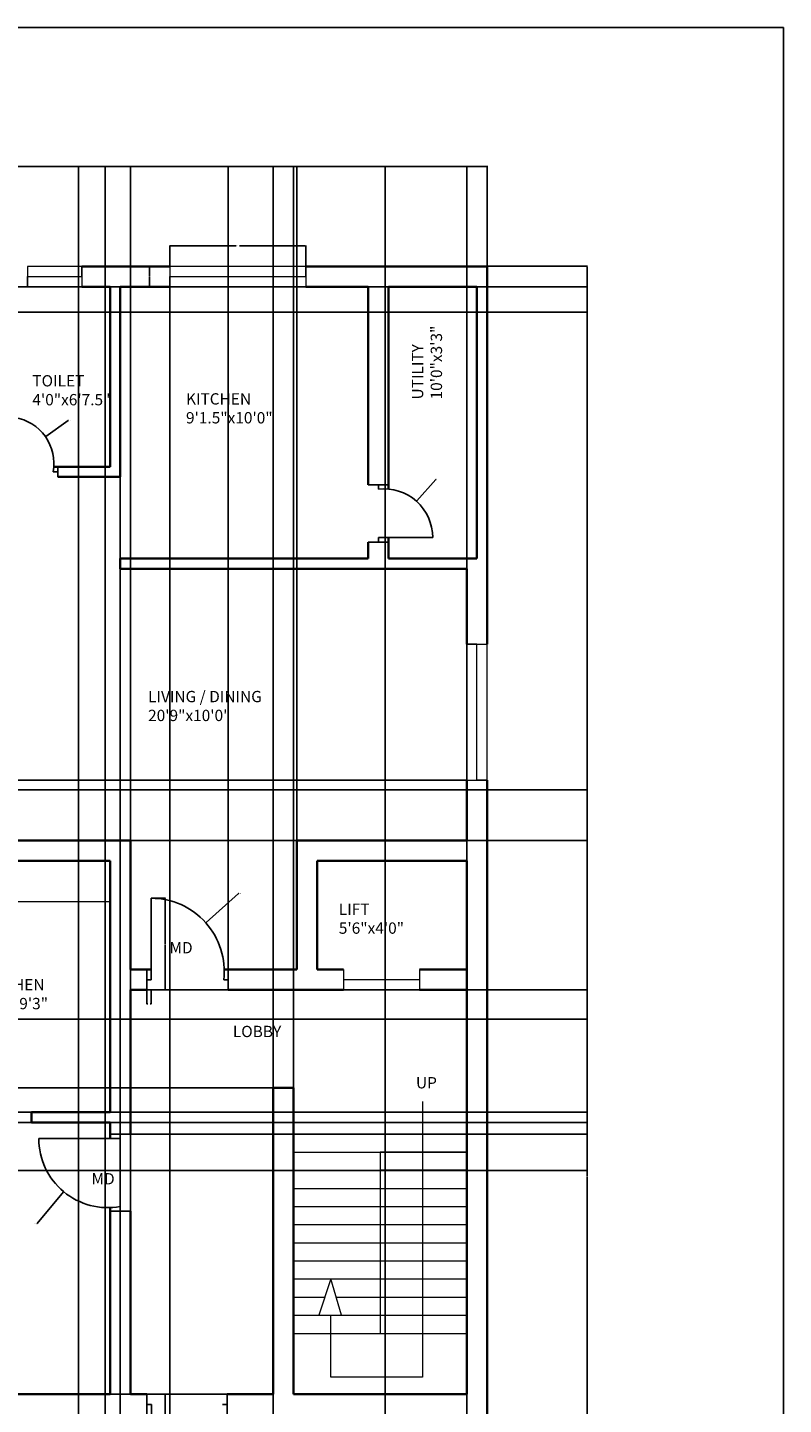
# Model space of a CAD drawing. Units: inches. Extents: x 1870 to 2611, y 1432 to 2511.
# Tile 5 of 5: x 2277 to 2611, y 1903 to 2511. Entities that reach past the tile are written whole.
import ezdxf

# ---------------------------------------------------------------- set-up
doc = ezdxf.new("R2010")
doc.units = ezdxf.units.IN
for name, color, linetype, lineweight in [('A-ANNO-DIMS', 2, 'Continuous', 18), ('A-ANNO-SYMB', 60, 'Continuous', 18), ('A-ANNO-TEXT', 7, 'Continuous', 18), ('A-ANNO-TTLB', 7, 'Continuous', 25), ('A-AREA-IDEN', 7, 'Continuous', 18), ('A-DOOR', 31, 'Continuous', 25), ('A-EQPM-ELEV', 4, 'Continuous', 18), ('A-FLOR-FIXT', 8, 'Continuous', 18), ('A-FLOR-STRS', 60, 'Continuous', 18), ('A-GLAZ', 201, 'Continuous', 18), ('A-WALL', 7, 'Continuous', 35)]:
    doc.layers.add(name, color=color, linetype=linetype, lineweight=lineweight)
doc.styles.get("Standard").update_dxf_attribs({"font": 'arial.ttf'})
doc.dimstyles.get("Standard").update_dxf_attribs({"dimtxt": 0.18, "dimasz": 0.18, "dimexe": 0.18, "dimexo": 0.0625, "dimgap": 0.09, "dimtad": 0, "dimtih": 1, "dimtoh": 1, "dimdec": 4, "dimzin": 0, "dimdsep": 46, "dimtxsty": 'Standard', "dimcen": 0.09, "dimadec": 0, "dimazin": 0, "dimtfac": 1, "dimtdec": 4, "dimtofl": 0, "dimtmove": 0, "dimatfit": 3, "dimfxl": 1, "dimtolj": 1, "dimtzin": 0, "dimarcsym": 0})

# ---------------------------------------------------------------- blocks, each defined once
blk = doc.blocks.new('DOOR-LEAF-36-JAMB-9-A')
for p, q in [((2, 4.5), (2, 40.5)), ((0, 9), (0, 0)), ((0, 0), (0, 4.5)), ((0, 4.5), (2, 4.5))]:
    blk.add_line(p, q)
blk = doc.blocks.new('DOOR-LEAF-36-JAMB-9-B')
for p, q in [((0, 40.5), (0, 31.5)), ((0, 31.5), (0, 36)), ((0, 36), (2, 36)), ((2, 36), (2, 0))]:
    blk.add_line(p, q)
blk = doc.blocks.new('WIN-60-FRAME-9')
for p, q in [((0, 9), (0, 0)), ((60, 9), (0, 9)), ((60, 4.5), (60, 9)), ((60, 9), (60, 0)), ((0, 0), (0, 4.5)), ((0, 4.5), (60, 4.5)), ((0, 0), (60, 0))]:
    blk.add_line(p, q)
blk = doc.blocks.new('WIN-24-FRAME-9')
for p, q in [((0, 9), (0, 0)), ((24, 9), (0, 9)), ((24, 4.5), (24, 9)), ((24, 9), (24, 0)), ((0, 0), (0, 4.5)), ((0, 4.5), (24, 4.5)), ((0, 0), (24, 0))]:
    blk.add_line(p, q)
blk = doc.blocks.new('*D11')
at = {"layer": 'A-ANNO-DIMS', "color": 0, "lineweight": -2, "transparency": 16777216}
for p, q in [((2340.04, 2405.43), (2340.04, 2414.55)), ((2340.22, 2414.37), (2369.28, 2414.37)), ((2399.86, 2414.37), (2370.79, 2414.37)), ((2400.04, 2405.43), (2400.04, 2414.55))]:
    blk.add_line(p, q, dxfattribs=at)
at = {"layer": 'A-ANNO-DIMS', "color": 0, "transparency": 16777216}
for points in [[(2340.22, 2414.4), (2340.22, 2414.34), (2340.04, 2414.37)], [(2399.86, 2414.4), (2399.86, 2414.34), (2400.04, 2414.37)]]:
    blk.add_solid(points, dxfattribs=at)
at = {"layer": 'Defpoints', "color": 0, "transparency": 16777216}
for p in [(2400.04, 2414.37), (2340.04, 2405.37), (2400.04, 2405.37)]:
    blk.add_point(p, dxfattribs=at)
at = {"layer": 'A-ANNO-DIMS', "color": 0, "transparency": 16777216, "insert": (2370.04, 2414.37), "char_height": 0.18, "attachment_point": 5}
blk.add_mtext('\\A1;W1 60 TYP.', dxfattribs=at)
blk = doc.blocks.new('*D12')
at = {"layer": 'A-ANNO-DIMS', "color": 0, "lineweight": -2, "transparency": 16777216}
for p, q in [((2339.97, 2405.37), (2330.86, 2405.37)), ((2331.04, 2405.19), (2331.04, 2401.05)), ((2339.97, 2396.37), (2330.86, 2396.37)), ((2331.04, 2396.55), (2331.04, 2400.69))]:
    blk.add_line(p, q, dxfattribs=at)
at = {"layer": 'A-ANNO-DIMS', "color": 0, "transparency": 16777216}
for points in [[(2331.01, 2405.19), (2331.07, 2405.19), (2331.04, 2405.37)], [(2331.01, 2396.55), (2331.07, 2396.55), (2331.04, 2396.37)]]:
    blk.add_solid(points, dxfattribs=at)
at = {"layer": 'Defpoints', "color": 0, "transparency": 16777216}
for p in [(2331.04, 2405.37), (2340.04, 2405.37), (2340.04, 2396.37)]:
    blk.add_point(p, dxfattribs=at)
at = {"layer": 'A-ANNO-DIMS', "color": 0, "transparency": 16777216, "insert": (2331.04, 2400.87), "char_height": 0.18, "attachment_point": 5}
blk.add_mtext('\\A1;9 TYP.', dxfattribs=at)
blk = doc.blocks.new('*D19')
at = {"layer": 'A-ANNO-DIMS', "color": 0, "lineweight": -2, "transparency": 16777216}
for p, q in [((2331.88, 2126.37), (2338.08, 2126.37)), ((2337.9, 2126.19), (2337.9, 2106.3)), ((2337.9, 2086.05), (2337.9, 2105.93)), ((2331.88, 2085.87), (2338.08, 2085.87))]:
    blk.add_line(p, q, dxfattribs=at)
at = {"layer": 'A-ANNO-DIMS', "color": 0, "transparency": 16777216}
for points in [[(2337.87, 2126.19), (2337.93, 2126.19), (2337.9, 2126.37)], [(2337.87, 2086.05), (2337.93, 2086.05), (2337.9, 2085.87)]]:
    blk.add_solid(points, dxfattribs=at)
at = {"layer": 'Defpoints', "color": 0, "transparency": 16777216}
for p in [(2331.82, 2126.37), (2337.9, 2126.37), (2331.82, 2085.87)]:
    blk.add_point(p, dxfattribs=at)
at = {"layer": 'A-ANNO-DIMS', "color": 0, "transparency": 16777216, "insert": (2337.9, 2106.12), "char_height": 0.18, "attachment_point": 5}
blk.add_mtext('\\A1;DOOR C 41 TYP.', dxfattribs=at)
blk = doc.blocks.new('*D20')
at = {"layer": 'A-ANNO-DIMS', "color": 0, "lineweight": -2, "transparency": 16777216}
for p, q in [((2329.82, 2085.8), (2329.82, 2079.61)), ((2331.82, 2085.8), (2331.82, 2079.61)), ((2330, 2079.79), (2330.36, 2079.79)), ((2331.64, 2079.79), (2331.28, 2079.79))]:
    blk.add_line(p, q, dxfattribs=at)
at = {"layer": 'A-ANNO-DIMS', "color": 0, "transparency": 16777216}
for points in [[(2330, 2079.82), (2330, 2079.76), (2329.82, 2079.79)], [(2331.64, 2079.82), (2331.64, 2079.76), (2331.82, 2079.79)]]:
    blk.add_solid(points, dxfattribs=at)
at = {"layer": 'Defpoints', "color": 0, "transparency": 16777216}
for p in [(2329.82, 2085.87), (2331.82, 2085.87), (2331.82, 2079.79)]:
    blk.add_point(p, dxfattribs=at)
at = {"layer": 'A-ANNO-DIMS', "color": 0, "transparency": 16777216, "insert": (2330.82, 2079.79), "char_height": 0.18, "attachment_point": 5}
blk.add_mtext('\\A1;2 TYP.', dxfattribs=at)
blk = doc.blocks.new('*D21')
at = {"layer": 'A-ANNO-DIMS', "color": 0, "lineweight": -2, "transparency": 16777216}
for p, q in [((2331.96, 1907.37), (2338.15, 1907.37)), ((2337.97, 1907.19), (2337.97, 1887.3)), ((2337.97, 1867.05), (2337.97, 1886.93)), ((2331.96, 1866.87), (2338.15, 1866.87))]:
    blk.add_line(p, q, dxfattribs=at)
at = {"layer": 'A-ANNO-DIMS', "color": 0, "transparency": 16777216}
for points in [[(2337.94, 1907.19), (2338, 1907.19), (2337.97, 1907.37)], [(2337.94, 1867.05), (2338, 1867.05), (2337.97, 1866.87)]]:
    blk.add_solid(points, dxfattribs=at)
at = {"layer": 'Defpoints', "color": 0, "transparency": 16777216}
for p in [(2331.9, 1907.37), (2337.97, 1907.37), (2331.9, 1866.87)]:
    blk.add_point(p, dxfattribs=at)
at = {"layer": 'A-ANNO-DIMS', "color": 0, "transparency": 16777216, "insert": (2337.97, 1887.12), "char_height": 0.18, "attachment_point": 5}
blk.add_mtext('\\A1;DOOR D 41 TYP.', dxfattribs=at)
blk = doc.blocks.new('*D25')
at = {"layer": 'A-ANNO-DIMS', "color": 0, "lineweight": -2, "transparency": 16777216}
for p, q in [((2004.64, 2405.43), (2004.64, 2449.7)), ((2004.82, 2449.52), (2241.99, 2449.52)), ((2479.96, 2449.52), (2242.78, 2449.52)), ((2480.14, 2405.43), (2480.14, 2449.7))]:
    blk.add_line(p, q, dxfattribs=at)
at = {"layer": 'A-ANNO-DIMS', "color": 0, "transparency": 16777216}
for points in [[(2004.82, 2449.55), (2004.82, 2449.49), (2004.64, 2449.52)], [(2479.96, 2449.55), (2479.96, 2449.49), (2480.14, 2449.52)]]:
    blk.add_solid(points, dxfattribs=at)
at = {"layer": 'Defpoints', "color": 0, "transparency": 16777216}
for p in [(2480.14, 2449.52), (2004.64, 2405.37), (2480.14, 2405.37)]:
    blk.add_point(p, dxfattribs=at)
at = {"layer": 'A-ANNO-DIMS', "color": 0, "transparency": 16777216, "insert": (2242.39, 2449.52), "char_height": 0.18, "attachment_point": 5}
blk.add_mtext('\\A1;475.5', dxfattribs=at)
blk = doc.blocks.new('*D26')
at = {"layer": 'A-ANNO-DIMS', "color": 0, "lineweight": -2, "transparency": 16777216}
for p, q in [((2480.2, 2405.37), (2524.47, 2405.37)), ((2524.29, 2405.19), (2524.29, 2003.55)), ((2524.29, 1601.55), (2524.29, 2003.19)), ((2480.2, 1601.37), (2524.47, 1601.37))]:
    blk.add_line(p, q, dxfattribs=at)
at = {"layer": 'A-ANNO-DIMS', "color": 0, "transparency": 16777216}
for points in [[(2524.26, 2405.19), (2524.32, 2405.19), (2524.29, 2405.37)], [(2524.26, 1601.55), (2524.32, 1601.55), (2524.29, 1601.37)]]:
    blk.add_solid(points, dxfattribs=at)
at = {"layer": 'Defpoints', "color": 0, "transparency": 16777216}
for p in [(2480.14, 2405.37), (2480.14, 1601.37), (2524.29, 1601.37)]:
    blk.add_point(p, dxfattribs=at)
at = {"layer": 'A-ANNO-DIMS', "color": 0, "transparency": 16777216, "insert": (2524.29, 2003.37), "char_height": 0.18, "attachment_point": 5}
blk.add_mtext('\\A1;804', dxfattribs=at)
blk = doc.blocks.new('*D33')
at = {"layer": 'A-ANNO-DIMS', "color": 0, "lineweight": -2, "transparency": 16777216}
for p, q in [((2394.64, 1907.43), (2394.64, 2449.7)), ((2394.82, 2449.52), (2432.56, 2449.52)), ((2470.96, 2449.52), (2433.21, 2449.52)), ((2471.14, 1907.43), (2471.14, 2449.7))]:
    blk.add_line(p, q, dxfattribs=at)
at = {"layer": 'A-ANNO-DIMS', "color": 0, "transparency": 16777216}
for points in [[(2394.82, 2449.55), (2394.82, 2449.49), (2394.64, 2449.52)], [(2470.96, 2449.55), (2470.96, 2449.49), (2471.14, 2449.52)]]:
    blk.add_solid(points, dxfattribs=at)
at = {"layer": 'Defpoints', "color": 0, "transparency": 16777216}
for p in [(2471.14, 2449.52), (2394.64, 1907.37), (2471.14, 1907.37)]:
    blk.add_point(p, dxfattribs=at)
at = {"layer": 'A-ANNO-DIMS', "color": 0, "transparency": 16777216, "insert": (2432.89, 2449.52), "char_height": 0.18, "attachment_point": 5}
blk.add_mtext('\\A1;76.5', dxfattribs=at)
blk = doc.blocks.new('*D34')
at = {"layer": 'A-ANNO-DIMS', "color": 0, "lineweight": -2, "transparency": 16777216}
for p, q in [((2385.57, 2042.61), (1960.31, 2042.61)), ((1960.49, 2042.43), (1960.49, 1975.17)), ((1960.49, 1907.55), (1960.49, 1974.8)), ((2385.57, 1907.37), (1960.31, 1907.37))]:
    blk.add_line(p, q, dxfattribs=at)
at = {"layer": 'A-ANNO-DIMS', "color": 0, "transparency": 16777216}
for points in [[(1960.46, 2042.43), (1960.52, 2042.43), (1960.49, 2042.61)], [(1960.46, 1907.55), (1960.52, 1907.55), (1960.49, 1907.37)]]:
    blk.add_solid(points, dxfattribs=at)
at = {"layer": 'Defpoints', "color": 0, "transparency": 16777216}
for p in [(1960.49, 2042.61), (2385.64, 2042.61), (2385.64, 1907.37)]:
    blk.add_point(p, dxfattribs=at)
at = {"layer": 'A-ANNO-DIMS', "color": 0, "transparency": 16777216, "insert": (1960.49, 1974.99), "char_height": 0.18, "attachment_point": 5}
blk.add_mtext('\\A1;135.24', dxfattribs=at)
blk = doc.blocks.new('*D35')
at = {"layer": 'A-ANNO-DIMS', "color": 0, "lineweight": -2, "transparency": 16777216}
for p, q in [((2322.64, 1907.43), (2322.64, 2449.7)), ((2322.82, 2449.52), (2353.92, 2449.52)), ((2385.46, 2449.52), (2354.36, 2449.52)), ((2385.64, 1907.43), (2385.64, 2449.7))]:
    blk.add_line(p, q, dxfattribs=at)
at = {"layer": 'A-ANNO-DIMS', "color": 0, "transparency": 16777216}
for points in [[(2322.82, 2449.55), (2322.82, 2449.49), (2322.64, 2449.52)], [(2385.46, 2449.55), (2385.46, 2449.49), (2385.64, 2449.52)]]:
    blk.add_solid(points, dxfattribs=at)
at = {"layer": 'Defpoints', "color": 0, "transparency": 16777216}
for p in [(2385.64, 2449.52), (2322.64, 1907.37), (2385.64, 1907.37)]:
    blk.add_point(p, dxfattribs=at)
at = {"layer": 'A-ANNO-DIMS', "color": 0, "transparency": 16777216, "insert": (2354.14, 2449.52), "char_height": 0.18, "attachment_point": 5}
blk.add_mtext('\\A1;63', dxfattribs=at)
blk = doc.blocks.new('*D36')
at = {"layer": 'A-ANNO-DIMS', "color": 0, "lineweight": -2, "transparency": 16777216}
for p, q in [((2365.82, 2094.93), (2365.82, 2449.7)), ((2366, 2449.52), (2380.6, 2449.52)), ((2395.96, 2449.52), (2381.36, 2449.52)), ((2396.14, 2094.93), (2396.14, 2449.7))]:
    blk.add_line(p, q, dxfattribs=at)
at = {"layer": 'A-ANNO-DIMS', "color": 0, "transparency": 16777216}
for points in [[(2366, 2449.55), (2366, 2449.49), (2365.82, 2449.52)], [(2395.96, 2449.55), (2395.96, 2449.49), (2396.14, 2449.52)]]:
    blk.add_solid(points, dxfattribs=at)
at = {"layer": 'Defpoints', "color": 0, "transparency": 16777216}
for p in [(2396.14, 2449.52), (2365.82, 2094.87), (2396.14, 2094.87)]:
    blk.add_point(p, dxfattribs=at)
at = {"layer": 'A-ANNO-DIMS', "color": 0, "transparency": 16777216, "insert": (2380.98, 2449.52), "char_height": 0.18, "attachment_point": 5}
blk.add_mtext('\\A1;30.31', dxfattribs=at)
blk = doc.blocks.new('*D37')
at = {"layer": 'A-ANNO-DIMS', "color": 0, "lineweight": -2, "transparency": 16777216}
for p, q in [((2322.7, 2085.87), (2524.47, 2085.87)), ((2524.29, 2085.69), (2524.29, 2054.24)), ((2524.29, 2022.42), (2524.29, 2053.87)), ((2322.7, 2022.24), (2524.47, 2022.24))]:
    blk.add_line(p, q, dxfattribs=at)
at = {"layer": 'A-ANNO-DIMS', "color": 0, "transparency": 16777216}
for points in [[(2524.26, 2085.69), (2524.32, 2085.69), (2524.29, 2085.87)], [(2524.26, 2022.42), (2524.32, 2022.42), (2524.29, 2022.24)]]:
    blk.add_solid(points, dxfattribs=at)
at = {"layer": 'Defpoints', "color": 0, "transparency": 16777216}
for p in [(2322.64, 2085.87), (2524.29, 2085.87), (2322.64, 2022.24)]:
    blk.add_point(p, dxfattribs=at)
at = {"layer": 'A-ANNO-DIMS', "color": 0, "transparency": 16777216, "insert": (2524.29, 2054.06), "char_height": 0.18, "attachment_point": 5}
blk.add_mtext('\\A1;63.62', dxfattribs=at)
blk = doc.blocks.new('*D38')
at = {"layer": 'A-ANNO-DIMS', "color": 0, "lineweight": -2, "transparency": 16777216}
for p, q in [((2385.64, 1907.3), (2385.64, 1485.35)), ((2365.31, 1898.3), (2365.31, 1485.35)), ((2365.49, 1485.53), (2375.01, 1485.53)), ((2385.46, 1485.53), (2375.94, 1485.53))]:
    blk.add_line(p, q, dxfattribs=at)
at = {"layer": 'A-ANNO-DIMS', "color": 0, "transparency": 16777216}
for points in [[(2365.49, 1485.56), (2365.49, 1485.5), (2365.31, 1485.53)], [(2385.46, 1485.56), (2385.46, 1485.5), (2385.64, 1485.53)]]:
    blk.add_solid(points, dxfattribs=at)
at = {"layer": 'Defpoints', "color": 0, "transparency": 16777216}
for p in [(2385.64, 1907.37), (2365.31, 1898.37), (2385.64, 1485.53)]:
    blk.add_point(p, dxfattribs=at)
at = {"layer": 'A-ANNO-DIMS', "color": 0, "transparency": 16777216, "insert": (2375.47, 1485.53), "char_height": 0.18, "attachment_point": 5}
blk.add_mtext('\\A1;20.328', dxfattribs=at)
blk = doc.blocks.new('*D42')
at = {"layer": 'A-ANNO-DIMS', "color": 0, "lineweight": -2, "transparency": 16777216}
for p, q in [((2318.14, 2396.3), (2318.14, 1485.35)), ((2340.04, 2396.3), (2340.04, 1485.35)), ((2318.32, 1485.53), (2328.76, 1485.53)), ((2339.86, 1485.53), (2329.41, 1485.53))]:
    blk.add_line(p, q, dxfattribs=at)
at = {"layer": 'A-ANNO-DIMS', "color": 0, "transparency": 16777216}
for points in [[(2318.32, 1485.56), (2318.32, 1485.5), (2318.14, 1485.53)], [(2339.86, 1485.56), (2339.86, 1485.5), (2340.04, 1485.53)]]:
    blk.add_solid(points, dxfattribs=at)
at = {"layer": 'Defpoints', "color": 0, "transparency": 16777216}
for p in [(2318.14, 2396.37), (2340.04, 2396.37), (2340.04, 1485.53)]:
    blk.add_point(p, dxfattribs=at)
at = {"layer": 'A-ANNO-DIMS', "color": 0, "transparency": 16777216, "insert": (2329.09, 1485.53), "char_height": 0.18, "attachment_point": 5}
blk.add_mtext('\\A1;21.9', dxfattribs=at)
blk = doc.blocks.new('*D46')
at = {"layer": 'A-ANNO-DIMS', "color": 0, "lineweight": -2, "transparency": 16777216}
for p, q in [((2299.67, 1649.43), (2299.67, 2449.7)), ((2299.85, 2449.52), (2305.14, 2449.52)), ((2311.34, 2449.52), (2306.05, 2449.52)), ((2311.52, 1649.43), (2311.52, 2449.7))]:
    blk.add_line(p, q, dxfattribs=at)
at = {"layer": 'A-ANNO-DIMS', "color": 0, "transparency": 16777216}
for points in [[(2299.85, 2449.55), (2299.85, 2449.49), (2299.67, 2449.52)], [(2311.34, 2449.55), (2311.34, 2449.49), (2311.52, 2449.52)]]:
    blk.add_solid(points, dxfattribs=at)
at = {"layer": 'Defpoints', "color": 0, "transparency": 16777216}
for p in [(2311.52, 2449.52), (2299.67, 1649.37), (2311.52, 1649.37)]:
    blk.add_point(p, dxfattribs=at)
at = {"layer": 'A-ANNO-DIMS', "color": 0, "transparency": 16777216, "insert": (2305.6, 2449.52), "char_height": 0.18, "attachment_point": 5}
blk.add_mtext('\\A1;11.846', dxfattribs=at)
blk = doc.blocks.new('*D47')
at = {"layer": 'A-ANNO-DIMS', "color": 0, "lineweight": -2, "transparency": 16777216}
for p, q in [((2435.2, 1649.43), (2435.2, 2449.7)), ((2435.38, 2449.52), (2452.77, 2449.52)), ((2470.96, 2449.52), (2453.56, 2449.52)), ((2471.14, 1649.43), (2471.14, 2449.7))]:
    blk.add_line(p, q, dxfattribs=at)
at = {"layer": 'A-ANNO-DIMS', "color": 0, "transparency": 16777216}
for points in [[(2435.38, 2449.55), (2435.38, 2449.49), (2435.2, 2449.52)], [(2470.96, 2449.55), (2470.96, 2449.49), (2471.14, 2449.52)]]:
    blk.add_solid(points, dxfattribs=at)
at = {"layer": 'Defpoints', "color": 0, "transparency": 16777216}
for p in [(2471.14, 2449.52), (2435.2, 1649.37), (2471.14, 1649.37)]:
    blk.add_point(p, dxfattribs=at)
at = {"layer": 'A-ANNO-DIMS', "color": 0, "transparency": 16777216, "insert": (2453.17, 2449.52), "char_height": 0.18, "attachment_point": 5}
blk.add_mtext('\\A1;35.94', dxfattribs=at)
blk = doc.blocks.new('*D48')
at = {"layer": 'A-ANNO-DIMS', "color": 0, "lineweight": -2, "transparency": 16777216}
for p, q in [((2471.07, 2178.54), (1960.31, 2178.54)), ((1960.49, 2178.36), (1960.49, 2165.39)), ((1960.49, 2152.05), (1960.49, 2165.02)), ((2471.07, 2151.87), (1960.31, 2151.87))]:
    blk.add_line(p, q, dxfattribs=at)
at = {"layer": 'A-ANNO-DIMS', "color": 0, "transparency": 16777216}
for points in [[(1960.46, 2178.36), (1960.52, 2178.36), (1960.49, 2178.54)], [(1960.46, 2152.05), (1960.52, 2152.05), (1960.49, 2151.87)]]:
    blk.add_solid(points, dxfattribs=at)
at = {"layer": 'Defpoints', "color": 0, "transparency": 16777216}
for p in [(1960.49, 2178.54), (2471.14, 2178.54), (2471.14, 2151.87)]:
    blk.add_point(p, dxfattribs=at)
at = {"layer": 'A-ANNO-DIMS', "color": 0, "transparency": 16777216, "insert": (1960.49, 2165.2), "char_height": 0.18, "attachment_point": 5}
blk.add_mtext('\\A1;26.673', dxfattribs=at)
blk = doc.blocks.new('*D51')
at = {"layer": 'A-ANNO-DIMS', "color": 0, "lineweight": -2, "transparency": 16777216}
for p, q in [((2013.7, 2072.92), (2524.47, 2072.92)), ((2524.29, 2072.74), (2524.29, 2052.57)), ((2524.29, 2032.05), (2524.29, 2052.21)), ((2013.7, 2031.87), (2524.47, 2031.87))]:
    blk.add_line(p, q, dxfattribs=at)
at = {"layer": 'A-ANNO-DIMS', "color": 0, "transparency": 16777216}
for points in [[(2524.26, 2072.74), (2524.32, 2072.74), (2524.29, 2072.92)], [(2524.26, 2032.05), (2524.32, 2032.05), (2524.29, 2031.87)]]:
    blk.add_solid(points, dxfattribs=at)
at = {"layer": 'Defpoints', "color": 0, "transparency": 16777216}
for p in [(2013.64, 2072.92), (2524.29, 2072.92), (2013.64, 2031.87)]:
    blk.add_point(p, dxfattribs=at)
at = {"layer": 'A-ANNO-DIMS', "color": 0, "transparency": 16777216, "insert": (2524.29, 2052.39), "char_height": 0.18, "attachment_point": 5}
blk.add_mtext('\\A1;41.05', dxfattribs=at)
blk = doc.blocks.new('*D52')
at = {"layer": 'A-ANNO-DIMS', "color": 0, "lineweight": -2, "transparency": 16777216}
for p, q in [((2052.7, 2396.37), (2524.47, 2396.37)), ((2524.29, 2396.19), (2524.29, 2390.94)), ((2524.29, 2385.32), (2524.29, 2390.57)), ((2052.7, 2385.14), (2524.47, 2385.14))]:
    blk.add_line(p, q, dxfattribs=at)
at = {"layer": 'A-ANNO-DIMS', "color": 0, "transparency": 16777216}
for points in [[(2524.26, 2396.19), (2524.32, 2396.19), (2524.29, 2396.37)], [(2524.26, 2385.32), (2524.32, 2385.32), (2524.29, 2385.14)]]:
    blk.add_solid(points, dxfattribs=at)
at = {"layer": 'Defpoints', "color": 0, "transparency": 16777216}
for p in [(2052.64, 2396.37), (2524.29, 2396.37), (2052.64, 2385.14)]:
    blk.add_point(p, dxfattribs=at)
at = {"layer": 'A-ANNO-DIMS', "color": 0, "transparency": 16777216, "insert": (2524.29, 2390.76), "char_height": 0.18, "attachment_point": 5}
blk.add_mtext('\\A1;11.223', dxfattribs=at)
blk = doc.blocks.new('*D53')
at = {"layer": 'A-ANNO-DIMS', "color": 0, "lineweight": -2, "transparency": 16777216}
for p, q in [((2052.7, 2174.24), (2524.47, 2174.24)), ((2524.29, 2174.06), (2524.29, 2163.24)), ((2524.29, 2152.05), (2524.29, 2162.87)), ((2052.7, 2151.87), (2524.47, 2151.87))]:
    blk.add_line(p, q, dxfattribs=at)
at = {"layer": 'A-ANNO-DIMS', "color": 0, "transparency": 16777216}
for points in [[(2524.26, 2174.06), (2524.32, 2174.06), (2524.29, 2174.24)], [(2524.26, 2152.05), (2524.32, 2152.05), (2524.29, 2151.87)]]:
    blk.add_solid(points, dxfattribs=at)
at = {"layer": 'Defpoints', "color": 0, "transparency": 16777216}
for p in [(2052.64, 2174.24), (2524.29, 2174.24), (2052.64, 2151.87)]:
    blk.add_point(p, dxfattribs=at)
at = {"layer": 'A-ANNO-DIMS', "color": 0, "transparency": 16777216, "insert": (2524.29, 2163.05), "char_height": 0.18, "attachment_point": 5}
blk.add_mtext('\\A1;22.376', dxfattribs=at)
blk = doc.blocks.new('*D54')
at = {"layer": 'A-ANNO-DIMS', "color": 0, "lineweight": -2, "transparency": 16777216}
for p, q in [((2074.58, 2027.37), (2524.47, 2027.37)), ((2524.29, 2027.19), (2524.29, 2016.94)), ((2524.29, 2006.33), (2524.29, 2016.58)), ((2074.58, 2006.15), (2524.47, 2006.15))]:
    blk.add_line(p, q, dxfattribs=at)
at = {"layer": 'A-ANNO-DIMS', "color": 0, "transparency": 16777216}
for points in [[(2524.26, 2027.19), (2524.32, 2027.19), (2524.29, 2027.37)], [(2524.26, 2006.33), (2524.32, 2006.33), (2524.29, 2006.15)]]:
    blk.add_solid(points, dxfattribs=at)
at = {"layer": 'Defpoints', "color": 0, "transparency": 16777216}
for p in [(2074.52, 2027.37), (2524.29, 2027.37), (2074.52, 2006.15)]:
    blk.add_point(p, dxfattribs=at)
at = {"layer": 'A-ANNO-DIMS', "color": 0, "transparency": 16777216, "insert": (2524.29, 2016.76), "char_height": 0.18, "attachment_point": 5}
blk.add_mtext('\\A1;21.215', dxfattribs=at)
blk = doc.blocks.new('*D58')
at = {"layer": 'A-ANNO-DIMS', "color": 0, "lineweight": -2, "transparency": 16777216}
for p, q in [((2370.36, 2128.4), (2356.04, 2115.67)), ((2370.54, 2128.4), (2370.36, 2128.4)), ((2331.73, 2094.14), (2331.91, 2094.14)), ((2331.82, 2094.05), (2331.82, 2094.23))]:
    blk.add_line(p, q, dxfattribs=at)
at = {"layer": 'A-ANNO-DIMS', "color": 0, "transparency": 16777216}
blk.add_solid([(2356.02, 2115.69), (2356.06, 2115.65), (2355.91, 2115.55)], dxfattribs=at)
at = {"layer": 'Defpoints', "color": 0, "transparency": 16777216}
for p in [(2355.91, 2115.55), (2331.82, 2094.14)]:
    blk.add_point(p, dxfattribs=at)
at = {"layer": 'A-ANNO-DIMS', "color": 0, "transparency": 16777216, "insert": (2371.09, 2128.4), "char_height": 0.18, "attachment_point": 5}
blk.add_mtext('\\A1;R32.225', dxfattribs=at)
blk = doc.blocks.new('*D60')
at = {"layer": 'A-ANNO-DIMS', "color": 0, "lineweight": -2, "transparency": 16777216}
for p, q in [((2312.53, 2020.24), (2312.71, 2020.24)), ((2312.62, 2020.15), (2312.62, 2020.33)), ((2281.41, 1982.77), (2293, 1996.68)), ((2281.23, 1982.77), (2281.41, 1982.77))]:
    blk.add_line(p, q, dxfattribs=at)
at = {"layer": 'A-ANNO-DIMS', "color": 0, "transparency": 16777216}
blk.add_solid([(2292.97, 1996.7), (2293.02, 1996.66), (2293.11, 1996.82)], dxfattribs=at)
at = {"layer": 'Defpoints', "color": 0, "transparency": 16777216}
for p in [(2312.62, 2020.24), (2293.11, 1996.82)]:
    blk.add_point(p, dxfattribs=at)
at = {"layer": 'A-ANNO-DIMS', "color": 0, "transparency": 16777216, "insert": (2280.75, 1982.77), "char_height": 0.18, "attachment_point": 5}
blk.add_mtext('\\A1;R30.48', dxfattribs=at)
blk = doc.blocks.new('*D67')
at = {"layer": 'A-ANNO-DIMS', "color": 0, "lineweight": -2, "transparency": 16777216}
for p, q in [((2457.49, 2311.3), (2449.05, 2301.81)), ((2457.67, 2311.3), (2457.49, 2311.3)), ((2434.56, 2285.62), (2434.74, 2285.62)), ((2434.65, 2285.53), (2434.65, 2285.71))]:
    blk.add_line(p, q, dxfattribs=at)
at = {"layer": 'A-ANNO-DIMS', "color": 0, "transparency": 16777216}
blk.add_solid([(2449.02, 2301.83), (2449.07, 2301.79), (2448.93, 2301.67)], dxfattribs=at)
at = {"layer": 'Defpoints', "color": 0, "transparency": 16777216}
for p in [(2448.93, 2301.67), (2434.65, 2285.62)]:
    blk.add_point(p, dxfattribs=at)
at = {"layer": 'A-ANNO-DIMS', "color": 0, "transparency": 16777216, "insert": (2458.22, 2311.3), "char_height": 0.18, "attachment_point": 5}
blk.add_mtext('\\A1;R21.483', dxfattribs=at)
blk = doc.blocks.new('*D68')
at = {"layer": 'A-ANNO-DIMS', "color": 0, "lineweight": -2, "transparency": 16777216}
for p, q in [((2295.13, 2337.35), (2285.2, 2330.3)), ((2295.31, 2337.35), (2295.13, 2337.35)), ((2268.18, 2318.28), (2268.36, 2318.28)), ((2268.27, 2318.19), (2268.27, 2318.37))]:
    blk.add_line(p, q, dxfattribs=at)
at = {"layer": 'A-ANNO-DIMS', "color": 0, "transparency": 16777216}
blk.add_solid([(2285.19, 2330.33), (2285.22, 2330.28), (2285.06, 2330.2)], dxfattribs=at)
at = {"layer": 'Defpoints', "color": 0, "transparency": 16777216}
for p in [(2285.06, 2330.2), (2268.27, 2318.28)]:
    blk.add_point(p, dxfattribs=at)
at = {"layer": 'A-ANNO-DIMS', "color": 0, "transparency": 16777216, "insert": (2295.86, 2337.35), "char_height": 0.18, "attachment_point": 5}
blk.add_mtext('\\A1;R20.593', dxfattribs=at)

msp = doc.modelspace()

# ---------------------------------------------------------------- linework, layer by layer
at = {"layer": 'A-ANNO-SYMB'}
for p, q in [((2451.6874, 2036.6327), (2451.6874, 1914.9725)), ((2411.1862, 1958.2645), (2405.8924, 1942.2645)), ((2415.8497, 1942.2645), (2411.1862, 1958.2645)), ((2405.8924, 1942.2645), (2415.8497, 1942.2645)), ((2411.1862, 1914.9725), (2411.1862, 1942.2645)), ((2451.6874, 1914.9725), (2411.1862, 1914.9725))]:
    msp.add_line(p, q, dxfattribs=at)
at = {"layer": 'A-ANNO-TTLB'}
msp.add_lwpolyline([(1869.7418, 2510.8018), (2611.0646, 2510.8018), (2611.0646, 1431.531), (1869.7418, 1431.531)], close=True, dxfattribs=at)
at = {"layer": 'A-DOOR'}
for p, q in [((2290.5308, 2316.8669), (2290.5308, 2312.3669)), ((2290.5308, 2314.6169), (2288.5308, 2314.6169)), ((2290.5308, 2312.3669), (2290.5308, 2314.6169)), ((2427.6359, 2308.9506), (2436.6359, 2308.9506)), ((2436.6359, 2308.9506), (2432.1359, 2308.9506)), ((2432.1359, 2308.9506), (2432.1359, 2306.9506)), ((2427.6359, 2283.6151), (2436.6359, 2283.6151)), ((2432.1359, 2283.6151), (2432.1359, 2285.6151)), ((2432.1359, 2285.6151), (2456.1359, 2285.6151)), ((2436.6359, 2283.6151), (2432.1359, 2283.6151)), ((2365.8249, 2094.8669), (2365.8249, 2085.8669)), ((2329.8215, 2090.3669), (2329.8215, 2090.3669)), ((2365.8249, 2090.3669), (2363.8249, 2090.3669)), ((2365.8249, 2085.8669), (2365.8249, 2090.3669)), ((2313.6359, 1988.267), (2322.6359, 1988.267)), ((2318.1359, 1988.267), (2318.1359, 1990.267)), ((2322.6359, 1988.267), (2318.1359, 1988.267)), ((2365.3084, 1902.8669), (2363.3084, 1902.8669)), ((2365.3084, 1898.3669), (2365.3084, 1907.3669)), ((2365.3084, 1907.3669), (2365.3084, 1902.8669))]:
    msp.add_line(p, q, dxfattribs=at)
for centre, radius, start, end in [((2268.2662, 2318.2782), 20.5927, 349.7587409, 80.9925275), ((2434.6525, 2285.6151), 21.4834, 360, 96.7270681), ((2331.8215, 2094.1417), 32.2252, 353.2731156, 90), ((2312.6174, 2020.2447), 30.4814, 180, 280.4307363)]:
    msp.add_arc(centre, radius, start, end, dxfattribs=at)
at = {"layer": 'A-EQPM-ELEV'}
for p, q in [((2416.6794, 2094.8669), (2416.6794, 2085.8669)), ((2450.3731, 2094.8669), (2450.3731, 2085.8669)), ((2450.3731, 2090.3669), (2416.6794, 2090.3669))]:
    msp.add_line(p, q, dxfattribs=at)
at = {"layer": 'A-FLOR-FIXT'}
msp.add_line((2228.9306, 2124.8754), (2313.6359, 2124.8754), dxfattribs=at)
at = {"layer": 'A-FLOR-STRS'}
for p, q in [((2394.6359, 2022.2645), (2471.1359, 2022.2645)), ((2394.6359, 2014.2645), (2471.1359, 2014.2645)), ((2471.1359, 2014.2645), (2432.8859, 2014.2645)), ((2432.8859, 2014.2645), (2432.8859, 1934.2645)), ((2394.6359, 2006.2645), (2471.1359, 2006.2645)), ((2471.1359, 2006.2645), (2432.8859, 2006.2645)), ((2394.6359, 1998.2645), (2471.1359, 1998.2645)), ((2394.6359, 1990.2645), (2471.1359, 1990.2645)), ((2394.6359, 1982.2645), (2471.1359, 1982.2645)), ((2394.6359, 1974.2645), (2471.1359, 1974.2645)), ((2394.6359, 1966.2645), (2471.1359, 1966.2645)), ((2394.6359, 1958.2645), (2471.1359, 1958.2645)), ((2394.6359, 1950.2645), (2408.5393, 1950.2645)), ((2413.518, 1950.2645), (2471.1359, 1950.2645)), ((2394.6359, 1942.2645), (2471.1359, 1942.2645)), ((2394.6359, 1934.2645), (2471.1359, 1934.2645))]:
    msp.add_line(p, q, dxfattribs=at)
at = {"layer": 'A-GLAZ'}
msp.add_line((2301.1709, 2405.3669), (2301.1709, 2405.3669), dxfattribs=at)
at = {"layer": 'A-WALL'}
for p, q in [((2301.1709, 2405.3669), (2340.0375, 2405.3669)), ((2301.1709, 2405.3669), (2340.0375, 2405.3669)), ((2400.0375, 2405.3669), (2480.1359, 2405.3669)), ((2400.0375, 2405.3669), (2480.1359, 2405.3669)), ((2480.1359, 2405.3669), (2480.1359, 2238.5402)), ((2301.1709, 2396.3669), (2313.6359, 2396.3669)), ((2313.6359, 2396.3669), (2313.6359, 2316.8669)), ((2318.1359, 2396.3669), (2318.1359, 2312.3669)), ((2318.1359, 2396.3669), (2340.0375, 2396.3669)), ((2400.0375, 2396.3669), (2427.6359, 2396.3669)), ((2427.6359, 2396.3669), (2427.6359, 2308.9506)), ((2436.6359, 2396.3669), (2436.6359, 2307.0068)), ((2436.6359, 2396.3669), (2475.6359, 2396.3669)), ((2475.6359, 2396.3669), (2475.6359, 2276.3669)), ((2288.8105, 2316.8669), (2313.6359, 2316.8669)), ((2290.5308, 2312.3669), (2318.1359, 2312.3669)), ((2427.6359, 2283.6151), (2427.6359, 2276.3669)), ((2436.6359, 2285.6151), (2436.6359, 2276.3669)), ((2318.1359, 2276.3669), (2427.6359, 2276.3669)), ((2318.1359, 2276.3669), (2318.1359, 2271.8669)), ((2436.6359, 2276.3669), (2475.6359, 2276.3669)), ((2318.1359, 2271.8669), (2471.1359, 2271.8669)), ((2471.1359, 2271.8669), (2471.1359, 2238.5402)), ((2471.1359, 2178.5402), (2471.1359, 2151.8669)), ((2480.1359, 2178.5402), (2480.1359, 1883.4206)), ((2052.6359, 2151.8669), (2322.6359, 2151.8669)), ((2322.6359, 2142.8669), (2322.6359, 2151.8669)), ((2396.1359, 2094.8669), (2396.1359, 2151.8669)), ((2396.1359, 2151.8669), (2471.1359, 2151.8669)), ((2214.6359, 2142.8669), (2313.6359, 2142.8669)), ((2313.6359, 2031.8669), (2313.6359, 2142.8669)), ((2322.6359, 2142.8669), (2322.6359, 2094.8669)), ((2471.1359, 2142.8669), (2405.1359, 2142.8669)), ((2405.1359, 2142.8669), (2405.1359, 2094.8669)), ((2405.1359, 2142.8669), (2471.1359, 2142.8669)), ((2471.1359, 2142.8669), (2471.1359, 1907.3669)), ((2322.6359, 2094.8669), (2331.8215, 2094.8669)), ((2364.0386, 2094.8669), (2396.1359, 2094.8669)), ((2405.1359, 2094.8669), (2416.6794, 2094.8669)), ((2450.3731, 2094.8669), (2471.1359, 2094.8669)), ((2471.1359, 2094.8669), (2471.1359, 2085.8669)), ((2329.8215, 2085.8669), (2322.6359, 2085.8669)), ((2322.6359, 2085.8669), (2322.6359, 2027.3669)), ((2396.1359, 2085.8669), (2365.8249, 2085.8669)), ((2405.1359, 2085.8669), (2396.1359, 2085.8669)), ((2396.1359, 2085.8669), (2396.1359, 2085.8669)), ((2416.6794, 2085.8669), (2405.1359, 2085.8669)), ((2471.1359, 2085.8669), (2450.3731, 2085.8669)), ((2394.6359, 2042.6068), (2385.6359, 2042.6068)), ((2385.6359, 2042.6068), (2385.6359, 1907.3669)), ((2394.6359, 1907.3669), (2394.6359, 2042.6068)), ((2278.8567, 2031.8669), (2278.8567, 2027.3669)), ((2278.8567, 2031.8669), (2313.6359, 2031.8669)), ((2278.8567, 2031.8669), (2313.6359, 2031.8669)), ((2278.8567, 2027.3669), (2313.6359, 2027.3669)), ((2313.6359, 2027.3669), (2313.6359, 2027.3669)), ((2313.6359, 2027.3669), (2313.6359, 2020.2447)), ((2322.6359, 2027.3669), (2322.6359, 2022.2447)), ((2313.6359, 1989.7803), (2313.6359, 1907.3669)), ((2322.6359, 1988.267), (2322.6359, 1907.3669)), ((2074.5182, 1907.3669), (2313.6359, 1907.3669)), ((2322.6359, 1907.3669), (2322.6359, 1907.3669)), ((2322.6359, 1907.3669), (2329.8969, 1907.3669)), ((2365.3084, 1907.3669), (2385.6359, 1907.3669)), ((2471.1359, 1907.3669), (2394.6359, 1907.3669)), ((2394.6359, 1907.3669), (2471.1359, 1907.3669))]:
    msp.add_line(p, q, dxfattribs=at)

# ---------------------------------------------------------------- block references
at = {"layer": 'A-DOOR'}
for name, p in [('DOOR-LEAF-36-JAMB-9-A', (2329.821, 2085.867)), ('DOOR-LEAF-36-JAMB-9-B', (2329.897, 1866.867))]:
    msp.add_blockref(name, p, dxfattribs=at)
at = {"layer": 'A-DOOR', "extrusion": (0, 0, -1), "zscale": -1, "rotation": 269.9999999999984}
msp.add_blockref('DOOR-LEAF-36-JAMB-9-A', (-2322.6359, 2022.2452), dxfattribs=at)
at = {"layer": 'A-GLAZ'}
for name, p in [('WIN-24-FRAME-9', (2277.171, 2396.367)), ('WIN-60-FRAME-9', (2340.0377, 2396.367))]:
    msp.add_blockref(name, p, dxfattribs=at)
at = {"layer": 'A-GLAZ', "rotation": 90.00000000000047}
msp.add_blockref('WIN-60-FRAME-9', (2480.1359, 2178.5404), dxfattribs=at)

# ---------------------------------------------------------------- texts
at = {"layer": 'A-ANNO-TEXT', "char_height": 5, "attachment_point": 1}
for s, width, insert in [('MD', 32.497853, (2339.8741, 2107.0408)), ('UP', 16.718552, (2448.7437, 2047.4117)), ('MD', 16.814932, (2305.4318, 2005.012))]:
    msp.add_mtext_dynamic_manual_height_columns(s, width=width, gutter_width=12.5, heights=[0], dxfattribs=dict(at, insert=insert))
at = {"layer": 'A-AREA-IDEN', "insert": (2446.9305, 2346.6), "char_height": 5, "attachment_point": 1, "rotation": 90}
msp.add_mtext_dynamic_manual_height_columns('UTILITY\\P10\'0"x3\'3"', width=126.135057, gutter_width=12.5, heights=[0], dxfattribs=at)
at = {"layer": 'A-AREA-IDEN', "char_height": 5, "attachment_point": 1}
for s, width, insert in [('TOILET\\P4\'0"x6\'7.5"', 28.096962, (2279.3023, 2357.3319)), ('KITCHEN\\P9\'1.5"x10\'0"', 111.841911, (2347.1629, 2349.3411)), ('LIVING / DINING\\P20\'9"x10\'0"', 171.698946, (2330.4267, 2217.9195)), ('LIFT\\P5\'6"x4\'0"', 65.463323, (2414.6726, 2124.0197)), ('KITCHEN\\P8\'3"x 9\'3"', 77.76941, (2255.9057, 2090.7047)), ('LOBBY', 51.470569, (2367.8636, 2070.0498))]:
    msp.add_mtext_dynamic_manual_height_columns(s, width=width, gutter_width=12.5, heights=[0], dxfattribs=dict(at, insert=insert))

# ---------------------------------------------------------------- dimensions: what is measured, and where the dimension line sits
at = {"layer": 'A-ANNO-DIMS'}
for base, p1, p2, override, picture, middle in [((2480.1359, 2449.5169), (2004.6359, 2405.3669), (2480.1359, 2405.3669), {"dimdec": 1, "dimlfac": 1, "dimrnd": 0, "dimzin": 0, "dimdsep": 46, "dimlunit": 2}, '*D25', (2242.3859, 2449.5169)), ((2311.5182, 2449.5169), (2299.6725, 1649.3669), (2311.5182, 1649.3669), {"dimdec": 3, "dimlfac": 1, "dimrnd": 0, "dimzin": 0, "dimdsep": 46, "dimlunit": 2}, '*D46', (2305.5954, 2449.5169)), ((2385.6359, 2449.5169), (2322.6359, 1907.3669), (2385.6359, 1907.3669), {"dimdec": 0, "dimlfac": 1, "dimrnd": 0, "dimzin": 0, "dimdsep": 46, "dimlunit": 2}, '*D35', (2354.1359, 2449.5169)), ((2396.1359, 2449.5169), (2365.8249, 2094.8669), (2396.1359, 2094.8669), {"dimdec": 2, "dimlfac": 1, "dimrnd": 0, "dimzin": 0, "dimdsep": 46, "dimlunit": 2}, '*D36', (2380.9804, 2449.5169)), ((2471.1359, 2449.5169), (2394.6359, 1907.3669), (2471.1359, 1907.3669), {"dimdec": 1, "dimlfac": 1, "dimrnd": 0, "dimzin": 0, "dimdsep": 46, "dimlunit": 2}, '*D33', (2432.8859, 2449.5169)), ((2471.1359, 2449.5169), (2435.1985, 1649.3669), (2471.1359, 1649.3669), {"dimdec": 2, "dimlfac": 1, "dimrnd": 0, "dimzin": 0, "dimdsep": 46, "dimlunit": 2}, '*D47', (2453.1672, 2449.5169)), ((2340.0375, 1485.5313), (2318.1359, 2396.3669), (2340.0375, 2396.3669), {"dimdec": 1, "dimlfac": 1, "dimrnd": 0, "dimzin": 0, "dimdsep": 46, "dimlunit": 2}, '*D42', (2329.0867, 1485.5313)), ((2385.63592, 1485.53127), (2365.30836, 1898.36694), (2385.63592, 1907.36694), {"dimdec": 3, "dimlfac": 1, "dimrnd": 0, "dimzin": 0, "dimdsep": 46, "dimlunit": 2}, '*D38', (2375.47214, 1485.53127))]:
    dim = msp.add_linear_dim(base=base, p1=p1, p2=p2, dimstyle='Standard', override=override, dxfattribs=at)
    dim.commit()
    dim.dimension.update_dxf_attribs({"geometry": picture, "text_midpoint": middle})
for base, p1, p2, text, picture, middle in [((2400.0375, 2414.3669), (2340.0375, 2405.3669), (2400.0375, 2405.3669), 'W1 <> TYP.', '*D11', (2370.0375, 2414.3669)), ((2331.8215, 2079.7919), (2329.8215, 2085.8669), (2331.8215, 2085.8669), '<> TYP.', '*D20', (2330.8215, 2079.7919))]:
    dim = msp.add_linear_dim(base=base, p1=p1, p2=p2, text=text, dimstyle='Standard', override={"dimdec": 0, "dimlfac": 1, "dimrnd": 0, "dimzin": 0, "dimdsep": 46, "dimlunit": 2}, dxfattribs=at)
    dim.commit()
    dim.dimension.update_dxf_attribs({"geometry": picture, "text_midpoint": middle})
for base, p1, p2, text, picture, middle in [((2331.0375, 2405.3669), (2340.0375, 2396.3669), (2340.0375, 2405.3669), '<> TYP.', '*D12', (2331.0375, 2400.8669)), ((2337.8964929321, 2126.3669377198), (2331.8214929321, 2085.8669377198), (2331.8214929321, 2126.3669377198), 'DOOR C <> TYP.', '*D19', (2337.8964929321, 2106.1169377198)), ((2337.9719273778, 1907.3669377198), (2331.8969273778, 1866.8669377198), (2331.8969273778, 1907.3669377198), 'DOOR D <> TYP.', '*D21', (2337.9719273778, 1887.1169377198))]:
    dim = msp.add_linear_dim(base=base, p1=p1, p2=p2, angle=90, text=text, dimstyle='Standard', override={"dimdec": 0, "dimlfac": 1, "dimrnd": 0, "dimzin": 0, "dimdsep": 46, "dimlunit": 2}, dxfattribs=at)
    dim.commit()
    dim.dimension.update_dxf_attribs({"geometry": picture, "text_midpoint": middle})
for base, p1, p2, override, picture, middle in [((2524.2859, 1601.3669), (2480.1359, 2405.3669), (2480.1359, 1601.3669), {"dimdec": 0, "dimlfac": 1, "dimrnd": 0, "dimzin": 0, "dimdsep": 46, "dimlunit": 2}, '*D26', (2524.2859, 2003.3669)), ((2524.2859, 2396.3669), (2052.6359, 2385.1438), (2052.6359, 2396.3669), {"dimdec": 3, "dimlfac": 1, "dimrnd": 0, "dimzin": 0, "dimdsep": 46, "dimlunit": 2}, '*D52', (2524.2859, 2390.7554)), ((1960.4859, 2178.5402), (2471.1359, 2151.8669), (2471.1359, 2178.5402), {"dimdec": 3, "dimlfac": 1, "dimrnd": 0, "dimzin": 0, "dimdsep": 46, "dimlunit": 2}, '*D48', (1960.4859, 2165.2036)), ((2524.2859, 2174.2429), (2052.6359, 2151.8669), (2052.6359, 2174.2429), {"dimdec": 3, "dimlfac": 1, "dimrnd": 0, "dimzin": 0, "dimdsep": 46, "dimlunit": 2}, '*D53', (2524.2859, 2163.0549)), ((2524.2859, 2085.8669), (2322.6359, 2022.2447), (2322.6359, 2085.8669), {"dimdec": 2, "dimlfac": 1, "dimrnd": 0, "dimzin": 0, "dimdsep": 46, "dimlunit": 2}, '*D37', (2524.2859, 2054.0558)), ((2524.2859, 2072.9155), (2013.6359, 2031.8669), (2013.6359, 2072.9155), {"dimdec": 2, "dimlfac": 1, "dimrnd": 0, "dimzin": 0, "dimdsep": 46, "dimlunit": 2}, '*D51', (2524.2859, 2052.3912)), ((1960.4859, 2042.6068), (2385.6359, 1907.3669), (2385.6359, 2042.6068), {"dimdec": 2, "dimlfac": 1, "dimrnd": 0, "dimzin": 0, "dimdsep": 46, "dimlunit": 2}, '*D34', (1960.4859, 1974.9869)), ((2524.2859, 2027.3669), (2074.5182, 2006.1522), (2074.5182, 2027.3669), {"dimdec": 3, "dimlfac": 1, "dimrnd": 0, "dimzin": 0, "dimdsep": 46, "dimlunit": 2}, '*D54', (2524.2859, 2016.7595))]:
    dim = msp.add_linear_dim(base=base, p1=p1, p2=p2, angle=90, dimstyle='Standard', override=override, dxfattribs=at)
    dim.commit()
    dim.dimension.update_dxf_attribs({"geometry": picture, "text_midpoint": middle})
for center, mpoint, override, picture, middle in [((2268.2662, 2318.2782), (2285.057, 2330.2), {"dimdec": 3, "dimlfac": 1, "dimrnd": 0, "dimzin": 0, "dimdsep": 46, "dimlunit": 2}, '*D68', (2295.8612, 2337.3531)), ((2434.6525, 2285.6151), (2448.9262, 2301.6712), {"dimdec": 3, "dimlfac": 1, "dimrnd": 0, "dimzin": 0, "dimdsep": 46, "dimlunit": 2}, '*D67', (2458.2202, 2311.3049)), ((2331.8215, 2094.1417), (2355.906, 2115.552), {"dimdec": 3, "dimlfac": 1, "dimrnd": 0, "dimzin": 0, "dimdsep": 46, "dimlunit": 2}, '*D58', (2371.0872, 2128.3982)), ((2312.6174, 2020.2447), (2293.1121, 1996.8212), {"dimdec": 2, "dimlfac": 1, "dimrnd": 0, "dimzin": 0, "dimdsep": 46, "dimlunit": 2}, '*D60', (2280.749, 1982.767))]:
    dim = msp.add_radius_dim(center=center, mpoint=mpoint, dimstyle='Standard', override=override, dxfattribs=at)
    dim.commit()
    dim.dimension.update_dxf_attribs({"geometry": picture, "text_midpoint": middle, "dimtype": 164})

doc.saveas('drawing.dxf')
